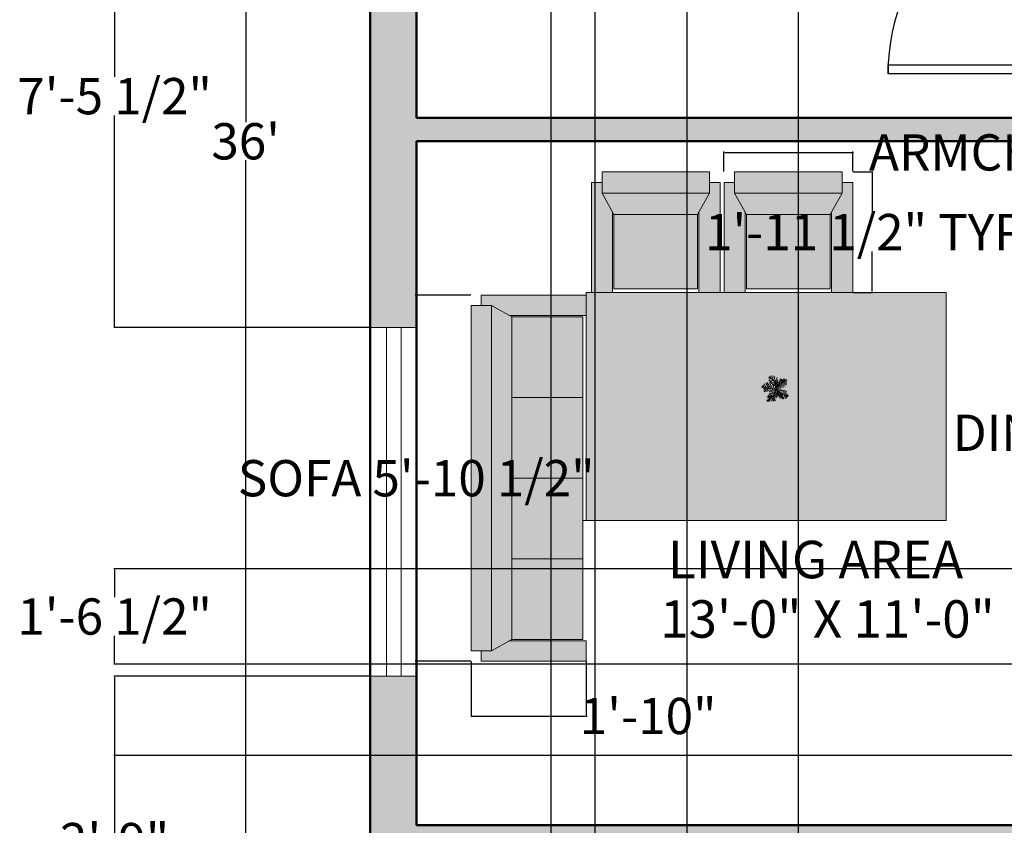
# Model space of a CAD drawing. Units: inches. Extents: x 2974 to 3443, y 2405 to 2963.
# Tile 2 of 13: x 2975 to 3165, y 2555 to 2711. Entities that reach past the tile are written whole.
import ezdxf

# ---------------------------------------------------------------- set-up
doc = ezdxf.new("R2010")
doc.units = ezdxf.units.IN
doc.header["$MEASUREMENT"] = 0
doc.layers.get('0').update_dxf_attribs({"color": 251})
for name, color, linetype, lineweight in [('A-ANNO-DIMS', 2, 'Continuous', 18), ('A-AREA-IDEN', 250, 'Continuous', 25), ('A-DOOR', 32, 'Continuous', 25), ('A-WALL-PATT', 252, 'Continuous', 13), ('furniture', 32, 'Continuous', 18), ('greenary', 106, 'Continuous', 13), ('walls', 250, 'Continuous', 50), ('windows', 159, 'Continuous', 20)]:
    doc.layers.add(name, color=color, linetype=linetype, lineweight=lineweight)
doc.layers.add('A-FURN-PATT', color=254, linetype='Continuous', lineweight=13, true_color=0xfeeab9)
doc.styles.get("Standard").update_dxf_attribs({"font": 'arial.ttf'})
doc.dimstyles.get("Standard").update_dxf_attribs({"dimtxt": 7, "dimasz": 0.18, "dimexe": 0.18, "dimexo": 0.0625, "dimgap": 0.09, "dimtad": 0, "dimtih": 1, "dimtoh": 1, "dimzin": 0, "dimdsep": 46, "dimlunit": 3, "dimtxsty": 'Standard', "dimcen": 0.09, "dimadec": 0, "dimazin": 0, "dimtfac": 1, "dimtofl": 0, "dimtmove": 0, "dimatfit": 3, "dimfxl": 1, "dimtolj": 1, "dimtzin": 0, "dimarcsym": 0})

# ---------------------------------------------------------------- blocks, each defined once
blk = doc.blocks.new('*U2')
for p, q in [((0, 0), (0, -6)), ((40, 0), (40, -6))]:
    blk.add_line(p, q)
blk.add_lwpolyline([(0, 0), (0, 40), (1.75, 40), (1.75, 0)], close=True)
blk.add_arc((0, 0), 40, 0, 90)
blk = doc.blocks.new('FABRIC SOFA 4S')
at = {"layer": 'furniture'}
for p, q in [((3, 54), (34, 54)), ((3, 51), (3, 54)), ((34, 48), (34, 54)), ((0, -51), (0, 51)), ((6, 51), (0, 51)), ((6, -51), (6, 51)), ((12, 47.63), (6, 51)), ((11.14, 48), (34, 48)), ((33, 23.81), (12, 23.81)), ((33, 0), (12, 0)), ((33, -23.81), (12, -23.81)), ((6, -51), (12, -47.63)), ((11.54, -48), (34, -48)), ((34, -48), (34, -54)), ((6, -51), (0, -51)), ((3, -54), (3, -51)), ((3, -54), (34, -54))]:
    blk.add_line(p, q, dxfattribs=at)
blk.add_lwpolyline([(12, -47.63), (12, 47.63), (33, 47.63), (33, -47.63)], close=True, dxfattribs=at)
blk = doc.blocks.new('FABRIC SOFA 1S')
at = {"layer": 'furniture'}
for p, q in [((3, 18.12), (34, 18.12)), ((3, 15.12), (3, 18.12)), ((34, 12.12), (34, 18.12)), ((0, -15.12), (0, 15.12)), ((6, 15.12), (0, 15.12)), ((6, -15.12), (6, 15.12)), ((12, 11.75), (6, 15.12)), ((11.33, 12.12), (34, 12.12)), ((6, -15.12), (12, -11.75)), ((11.33, -12.12), (34, -12.12)), ((34, -12.12), (34, -18.12)), ((6, -15.12), (0, -15.12)), ((3, -18.12), (3, -15.12)), ((3, -18.12), (34, -18.12))]:
    blk.add_line(p, q, dxfattribs=at)
blk.add_lwpolyline([(12, -11.75), (12, 11.75), (33, 11.75), (33, -11.75)], close=True, dxfattribs=at)
blk = doc.blocks.new('*U13')
for p, q in [((-5.114, 28.097), (-24.676, 40.636)), ((-7.288, 39.707), (-21.778, 46.673)), ((-8.737, 47.138), (-17.069, 52.711)), ((-10.186, 53.64), (-13.084, 55.962)), ((0, 0), (-10.5, 57)), ((-9.099, 51.782), (-6.563, 55.962)), ((-7.65, 43.423), (-2.578, 49.46)), ((-5.839, 35.992), (4.667, 48.067)), ((-5.114, 27.632), (10.463, 46.673)), ((-47.498, 19.737), (-55.83, 18.344)), ((-40.615, 13.7), (-55.105, 10.913)), ((-31.5, 4.5), (-52.5, 25.5)), ((-33.37, 6.269), (-52.207, 5.34)), ((-48.585, 21.131), (-49.309, 29.026)), ((-28.299, 3.483), (-47.86, -5.805)), ((-43.513, 28.561), (-42.427, 15.558)), ((-38.442, 26.239), (-34.819, 7.663)), ((-21.416, 3.018), (-38.079, -8.128)), ((-35.544, 28.097), (-24.314, 3.947)), ((0, 0), (-31.5, 4.5)), ((-14.533, 2.09), (-30.834, 25.31)), ((-15.982, 2.09), (-30.11, -9.521)), ((-3.665, 19.273), (-27.574, 35.527)), ((-24.314, 23.917), (-2.941, 13.7)), ((0, 0), (-22.5, -19.5)), ((-6.563, 1.161), (-21.416, -8.128)), ((-20.691, 13.7), (-1.129, 4.876)), ((-2.941, 16.486), (8.652, 37.85)), ((-1.129, 6.734), (9.014, 26.704)), ((0, 0), (27, 9)), ((0, 0), (18, -22.5)), ((3.942, 1.625), (11.187, 24.381)), ((6.478, 1.625), (26.04, -8.592)), ((10.101, 3.483), (17.708, 26.239)), ((11.187, 3.483), (30.749, -5.805)), ((16.259, 5.805), (23.142, 31.348)), ((18.07, 5.805), (35.096, -3.483)), ((22.055, 7.198), (27.489, 32.277)), ((24.229, 7.663), (46.688, 1.625)), ((27, 9), (48, 36)), ((27.127, 9.056), (31.112, 35.992)), ((29.662, 12.307), (48.137, 6.269)), ((31.836, 30.883), (32.561, 16.486)), ((33.285, 16.486), (48.862, 10.913)), ((35.096, 32.741), (37.27, 22.524)), ((36.183, 19.737), (48.137, 17.88)), ((38.719, 34.134), (41.979, 28.561)), ((40.53, 25.775), (48.862, 24.846)), ((43.791, 29.954), (51.036, 30.883)), ((44.153, 36.456), (45.239, 32.741)), ((-17.431, -15.094), (-42.789, -18.809)), ((-28.299, -29.026), (-42.789, -31.348)), ((-24.314, -21.596), (-42.427, -22.06)), ((-30.834, -34.135), (-42.427, -35.528)), ((-34.457, -39.708), (-40.978, -42.494)), ((-26.849, -26.24), (-40.253, -25.775)), ((-22.5, -19.5), (-37.5, -45)), ((-32.646, -36.921), (-31.921, -44.352)), ((-15.257, -12.772), (-30.11, -12.772)), ((-29.023, -30.884), (-27.936, -43.887)), ((-25.038, -23.918), (-22.865, -45.281)), ((-20.691, -18.345), (-17.793, -44.352)), ((-6.563, -5.805), (-19.967, -9.985)), ((-17.069, -15.094), (-12.721, -40.172)), ((-13.446, -11.378), (-8.737, -32.741)), ((-9.461, -8.592), (-6.201, -23.453)), ((-4.752, -3.483), (-3.665, -14.629)), ((2.493, -3.019), (-1.491, -20.202)), ((1.769, -2.555), (24.229, -9.521)), ((5.029, -6.27), (2.131, -25.775)), ((9.014, -11.378), (3.58, -35.992)), ((14.085, -16.951), (6.478, -40.172)), ((7.565, -9.056), (32.198, -14.629)), ((18.07, -22.524), (8.289, -45.745)), ((12.274, -15.094), (36.907, -18.809)), ((20.244, -30.419), (15.897, -44.816)), ((16.259, -19.738), (36.183, -22.989)), ((18, -22.5), (27, -52.5)), ((18.433, -22.524), (40.53, -29.026)), ((19.157, -25.311), (38.719, -33.206)), ((22.78, -37.85), (19.519, -48.532)), ((21.331, -32.741), (39.081, -40.636)), ((22.78, -38.314), (34.372, -44.816)), ((24.591, -45.745), (23.142, -50.854)), ((24.591, -43.423), (30.749, -47.603)), ((26.764, -49.925), (28.213, -50.854))]:
    blk.add_line(p, q)
blk = doc.blocks.new('*D20')
at = {"layer": 'A-ANNO-DIMS', "color": 0, "lineweight": -2, "transparency": 16777216}
for p, q in [((3018.41, 2903.19), (3018.14, 2903.19)), ((3018.32, 2903.01), (3018.32, 2690.85)), ((3018.32, 2471.37), (3018.32, 2683.52)), ((3018.41, 2471.19), (3018.14, 2471.19))]:
    blk.add_line(p, q, dxfattribs=at)
at = {"layer": 'A-ANNO-DIMS', "color": 0, "transparency": 16777216}
for points in [[(3018.29, 2903.01), (3018.35, 2903.01), (3018.32, 2903.19)], [(3018.29, 2471.37), (3018.35, 2471.37), (3018.32, 2471.19)]]:
    blk.add_solid(points, dxfattribs=at)
at = {"layer": 'Defpoints', "color": 0, "transparency": 16777216}
for p in [(3018.47, 2903.19), (3018.32, 2471.19), (3018.47, 2471.19)]:
    blk.add_point(p, dxfattribs=at)
at = {"layer": 'A-ANNO-DIMS', "color": 0, "transparency": 16777216, "insert": (3018.32, 2687.19), "char_height": 7, "attachment_point": 5}
blk.add_mtext("\\A1;36'", dxfattribs=at)
blk = doc.blocks.new('WIN-67IN')
for p, q in [((0, 0), (9, 0)), ((0, -67.29), (0, 0)), ((0, 0), (3.19, 0)), ((3.19, 0), (3.19, -67.29)), ((6.02, -67.29), (6.02, 0)), ((9, 0), (9, -67.29)), ((9, -67.29), (0, -67.29)), ((3.19, -67.29), (6.02, -67.29))]:
    blk.add_line(p, q)
blk = doc.blocks.new('*D35')
at = {"layer": 'A-ANNO-DIMS', "color": 0, "lineweight": -2, "transparency": 16777216}
for p, q in [((3110.66, 2681.38), (3110.66, 2685.22)), ((3110.84, 2685.04), (3135.33, 2685.04)), ((3135.51, 2681.38), (3135.51, 2685.22)), ((3135.51, 2685.04), (3135.69, 2685.04))]:
    blk.add_line(p, q, dxfattribs=at)
at = {"layer": 'A-ANNO-DIMS', "color": 0, "transparency": 16777216}
for points in [[(3110.84, 2685.07), (3110.84, 2685.01), (3110.66, 2685.04)], [(3135.33, 2685.07), (3135.33, 2685.01), (3135.51, 2685.04)]]:
    blk.add_solid(points, dxfattribs=at)
at = {"layer": 'Defpoints', "color": 0, "transparency": 16777216}
for p in [(3135.51, 2685.04), (3110.66, 2681.32), (3135.51, 2681.32)]:
    blk.add_point(p, dxfattribs=at)
at = {"layer": 'A-ANNO-DIMS', "color": 0, "transparency": 16777216, "insert": (3184.75, 2685.04), "char_height": 7, "attachment_point": 5}
blk.add_mtext('\\A1;ARMCHAIR 2\'-1" TYP.', dxfattribs=at)
blk = doc.blocks.new('*D36')
at = {"layer": 'A-ANNO-DIMS', "color": 0, "lineweight": -2, "transparency": 16777216}
for p, q in [((3135.57, 2681.32), (3139.42, 2681.32)), ((3139.24, 2681.14), (3139.24, 2673.37)), ((3139.24, 2658.19), (3139.24, 2665.95)), ((3135.57, 2658.01), (3139.42, 2658.01))]:
    blk.add_line(p, q, dxfattribs=at)
at = {"layer": 'A-ANNO-DIMS', "color": 0, "transparency": 16777216}
for points in [[(3139.21, 2681.14), (3139.27, 2681.14), (3139.24, 2681.32)], [(3139.21, 2658.19), (3139.27, 2658.19), (3139.24, 2658.01)]]:
    blk.add_solid(points, dxfattribs=at)
at = {"layer": 'Defpoints', "color": 0, "transparency": 16777216}
for p in [(3135.51, 2681.32), (3135.51, 2658.01), (3139.24, 2658.01)]:
    blk.add_point(p, dxfattribs=at)
at = {"layer": 'A-ANNO-DIMS', "color": 0, "transparency": 16777216, "insert": (3139.24, 2669.66), "char_height": 7, "attachment_point": 5}
blk.add_mtext('\\A1;1\'-11 1/2" TYP.', dxfattribs=at)
blk = doc.blocks.new('*D47')
at = {"layer": 'A-ANNO-DIMS', "color": 0, "lineweight": -2, "transparency": 16777216}
for p, q in [((3247.43, 2644.02), (3247.43, 2630.76)), ((3334.99, 2644.02), (3334.99, 2630.76)), ((3247.43, 2630.94), (3247.25, 2630.94)), ((3334.81, 2630.94), (3247.61, 2630.94))]:
    blk.add_line(p, q, dxfattribs=at)
at = {"layer": 'A-ANNO-DIMS', "color": 0, "transparency": 16777216}
for points in [[(3247.61, 2630.97), (3247.61, 2630.91), (3247.43, 2630.94)], [(3334.81, 2630.97), (3334.81, 2630.91), (3334.99, 2630.94)]]:
    blk.add_solid(points, dxfattribs=at)
at = {"layer": 'Defpoints', "color": 0, "transparency": 16777216}
for p in [(3247.43, 2644.08), (3334.99, 2644.08), (3247.43, 2630.94)]:
    blk.add_point(p, dxfattribs=at)
at = {"layer": 'A-ANNO-DIMS', "color": 0, "transparency": 16777216, "insert": (3200.53, 2630.94), "char_height": 7, "attachment_point": 5}
blk.add_mtext('\\A1;DINING SET 7\'-3 1/2"', dxfattribs=at)
blk = doc.blocks.new('*D49')
at = {"layer": 'A-ANNO-DIMS', "color": 0, "lineweight": -2, "transparency": 16777216}
for p, q in [((3061.77, 2657.48), (3051.06, 2657.48)), ((3051.24, 2657.3), (3051.24, 2625.89)), ((3051.24, 2587.05), (3051.24, 2618.46)), ((3061.77, 2586.87), (3051.06, 2586.87))]:
    blk.add_line(p, q, dxfattribs=at)
at = {"layer": 'A-ANNO-DIMS', "color": 0, "transparency": 16777216}
for points in [[(3051.21, 2657.3), (3051.27, 2657.3), (3051.24, 2657.48)], [(3051.21, 2587.05), (3051.27, 2587.05), (3051.24, 2586.87)]]:
    blk.add_solid(points, dxfattribs=at)
at = {"layer": 'Defpoints', "color": 0, "transparency": 16777216}
for p in [(3061.83, 2657.48), (3051.24, 2586.87), (3061.83, 2586.87)]:
    blk.add_point(p, dxfattribs=at)
at = {"layer": 'A-ANNO-DIMS', "color": 0, "transparency": 16777216, "insert": (3051.24, 2622.17), "char_height": 7, "attachment_point": 5}
blk.add_mtext('\\A1;SOFA 5\'-10 1/2"', dxfattribs=at)
blk = doc.blocks.new('*D50')
at = {"layer": 'A-ANNO-DIMS', "color": 0, "lineweight": -2, "transparency": 16777216}
for p, q in [((3061.83, 2586.81), (3061.83, 2576.1)), ((3084.06, 2586.81), (3084.06, 2576.1)), ((3062.01, 2576.28), (3083.88, 2576.28)), ((3084.06, 2576.28), (3084.24, 2576.28))]:
    blk.add_line(p, q, dxfattribs=at)
at = {"layer": 'A-ANNO-DIMS', "color": 0, "transparency": 16777216}
for points in [[(3062.01, 2576.31), (3062.01, 2576.25), (3061.83, 2576.28)], [(3083.88, 2576.31), (3083.88, 2576.25), (3084.06, 2576.28)]]:
    blk.add_solid(points, dxfattribs=at)
at = {"layer": 'Defpoints', "color": 0, "transparency": 16777216}
for p in [(3061.83, 2586.87), (3084.06, 2586.87), (3084.06, 2576.28)]:
    blk.add_point(p, dxfattribs=at)
at = {"layer": 'A-ANNO-DIMS', "color": 0, "transparency": 16777216, "insert": (3096.02, 2576.28), "char_height": 7, "attachment_point": 5}
blk.add_mtext('\\A1;1\'-10"', dxfattribs=at)
blk = doc.blocks.new('*D54')
at = {"layer": 'A-ANNO-DIMS', "color": 0, "lineweight": -2, "transparency": 16777216}
for p, q in [((3042.26, 2583.94), (2992.84, 2583.94)), ((2993.02, 2583.76), (2993.02, 2531.23)), ((2993.02, 2471.37), (2993.02, 2523.9)), ((3042.26, 2471.19), (2992.84, 2471.19))]:
    blk.add_line(p, q, dxfattribs=at)
at = {"layer": 'A-ANNO-DIMS', "color": 0, "transparency": 16777216}
for points in [[(2992.99, 2583.76), (2993.05, 2583.76), (2993.02, 2583.94)], [(2992.99, 2471.37), (2993.05, 2471.37), (2993.02, 2471.19)]]:
    blk.add_solid(points, dxfattribs=at)
at = {"layer": 'Defpoints', "color": 0, "transparency": 16777216}
for p in [(2993.02, 2583.94), (3042.33, 2583.94), (3042.33, 2471.19)]:
    blk.add_point(p, dxfattribs=at)
at = {"layer": 'A-ANNO-DIMS', "color": 0, "transparency": 16777216, "insert": (2993.02, 2527.57), "char_height": 7, "attachment_point": 5}
blk.add_mtext('\\A1;9\'-5"', dxfattribs=at)
blk = doc.blocks.new('*D55')
at = {"layer": 'A-ANNO-DIMS', "color": 0, "lineweight": -2, "transparency": 16777216}
for p, q in [((3042.26, 2740.57), (2992.84, 2740.57)), ((2993.02, 2740.39), (2993.02, 2699.61)), ((2993.02, 2651.41), (2993.02, 2692.19)), ((3042.26, 2651.23), (2992.84, 2651.23))]:
    blk.add_line(p, q, dxfattribs=at)
at = {"layer": 'A-ANNO-DIMS', "color": 0, "transparency": 16777216}
for points in [[(2992.99, 2740.39), (2993.05, 2740.39), (2993.02, 2740.57)], [(2992.99, 2651.41), (2993.05, 2651.41), (2993.02, 2651.23)]]:
    blk.add_solid(points, dxfattribs=at)
at = {"layer": 'Defpoints', "color": 0, "transparency": 16777216}
for p in [(3042.33, 2740.57), (2993.02, 2651.23), (3042.33, 2651.23)]:
    blk.add_point(p, dxfattribs=at)
at = {"layer": 'A-ANNO-DIMS', "color": 0, "transparency": 16777216, "insert": (2993.02, 2695.9), "char_height": 7, "attachment_point": 5}
blk.add_mtext('\\A1;7\'-5 1/2"', dxfattribs=at)
blk = doc.blocks.new('*D64')
at = {"layer": 'A-ANNO-DIMS', "color": 0, "lineweight": -2, "transparency": 16777216}
for p, q in [((3103.48, 2840.13), (3103.48, 2414.92)), ((3124.99, 2840.13), (3124.99, 2414.92)), ((3103.66, 2415.1), (3124.81, 2415.1)), ((3124.99, 2415.1), (3125.17, 2415.1))]:
    blk.add_line(p, q, dxfattribs=at)
at = {"layer": 'A-ANNO-DIMS', "color": 0, "transparency": 16777216}
for points in [[(3103.66, 2415.13), (3103.66, 2415.07), (3103.48, 2415.1)], [(3124.81, 2415.13), (3124.81, 2415.07), (3124.99, 2415.1)]]:
    blk.add_solid(points, dxfattribs=at)
at = {"layer": 'Defpoints', "color": 0, "transparency": 16777216}
for p in [(3103.48, 2840.19), (3124.99, 2840.19), (3124.99, 2415.1)]:
    blk.add_point(p, dxfattribs=at)
at = {"layer": 'A-ANNO-DIMS', "color": 0, "transparency": 16777216, "insert": (3142.39, 2415.1), "char_height": 7, "attachment_point": 5}
blk.add_mtext('\\A1;1\'-9 1/2"', dxfattribs=at)
blk = doc.blocks.new('*D68')
at = {"layer": 'A-ANNO-DIMS', "color": 0, "lineweight": -2, "transparency": 16777216}
for p, q in [((3077.27, 2480.25), (3077.27, 2952.68)), ((3077.45, 2952.5), (3085.63, 2952.5)), ((3085.81, 2480.25), (3085.81, 2952.68)), ((3085.81, 2952.5), (3085.99, 2952.5))]:
    blk.add_line(p, q, dxfattribs=at)
at = {"layer": 'A-ANNO-DIMS', "color": 0, "transparency": 16777216}
for points in [[(3077.45, 2952.53), (3077.45, 2952.47), (3077.27, 2952.5)], [(3085.63, 2952.53), (3085.63, 2952.47), (3085.81, 2952.5)]]:
    blk.add_solid(points, dxfattribs=at)
at = {"layer": 'Defpoints', "color": 0, "transparency": 16777216}
for p in [(3085.81, 2952.5), (3077.27, 2480.19), (3085.81, 2480.19)]:
    blk.add_point(p, dxfattribs=at)
at = {"layer": 'A-ANNO-DIMS', "color": 0, "transparency": 16777216, "insert": (3103.54, 2952.5), "char_height": 7, "attachment_point": 5}
blk.add_mtext('\\A1;0\'-8 1/2"', dxfattribs=at)
blk = doc.blocks.new('*D73')
at = {"layer": 'A-ANNO-DIMS', "color": 0, "lineweight": -2, "transparency": 16777216}
for p, q in [((3329.94, 2604.69), (2992.84, 2604.69)), ((2993.02, 2604.51), (2993.02, 2599.19)), ((2993.02, 2586.45), (2993.02, 2591.77)), ((3330, 2586.27), (2992.84, 2586.27))]:
    blk.add_line(p, q, dxfattribs=at)
at = {"layer": 'A-ANNO-DIMS', "color": 0, "transparency": 16777216}
for points in [[(2992.99, 2604.51), (2993.05, 2604.51), (2993.02, 2604.69)], [(2992.99, 2586.45), (2993.05, 2586.45), (2993.02, 2586.27)]]:
    blk.add_solid(points, dxfattribs=at)
at = {"layer": 'Defpoints', "color": 0, "transparency": 16777216}
for p in [(2993.02, 2604.69), (3330, 2604.69), (3330.06, 2586.27)]:
    blk.add_point(p, dxfattribs=at)
at = {"layer": 'A-ANNO-DIMS', "color": 0, "transparency": 16777216, "insert": (2993.02, 2595.48), "char_height": 7, "attachment_point": 5}
blk.add_mtext('\\A1;1\'-6 1/2"', dxfattribs=at)
blk = doc.blocks.new('*D76')
at = {"layer": 'A-ANNO-DIMS', "color": 0, "lineweight": -2, "transparency": 16777216}
for p, q in [((3352.84, 2568.64), (2992.84, 2568.64)), ((2993.02, 2568.46), (2993.02, 2555.8)), ((2993.02, 2535.82), (2993.02, 2548.48)), ((3352.84, 2535.64), (2992.84, 2535.64))]:
    blk.add_line(p, q, dxfattribs=at)
at = {"layer": 'A-ANNO-DIMS', "color": 0, "transparency": 16777216}
for points in [[(2992.99, 2568.46), (2993.05, 2568.46), (2993.02, 2568.64)], [(2992.99, 2535.82), (2993.05, 2535.82), (2993.02, 2535.64)]]:
    blk.add_solid(points, dxfattribs=at)
at = {"layer": 'Defpoints', "color": 0, "transparency": 16777216}
for p in [(2993.02, 2568.64), (3352.9, 2568.64), (3352.9, 2535.64)]:
    blk.add_point(p, dxfattribs=at)
at = {"layer": 'A-ANNO-DIMS', "color": 0, "transparency": 16777216, "insert": (2993.02, 2552.14), "char_height": 7, "attachment_point": 5}
blk.add_mtext('\\A1;2\'-9"', dxfattribs=at)

msp = doc.modelspace()

# ---------------------------------------------------------------- hatches: boundary and pattern name
at = {"layer": 'A-FURN-PATT'}
h = msp.add_hatch(color=256, dxfattribs=at)
h.dxf.hatch_style = 1
h.paths.add_polyline_path([(3105.53, 2673.089), (3089.42, 2673.089), (3089.42, 2658.693), (3105.53, 2658.693)])
h.paths.add_polyline_path([(3089.163, 2673.546), (3087.106, 2677.202), (3087.106, 2679.259), (3085.05, 2679.259), (3085.05, 2658.007), (3089.163, 2658.007)])
h.paths.add_polyline_path([(3109.901, 2679.259), (3107.844, 2679.259), (3107.844, 2677.202), (3105.787, 2673.546), (3105.787, 2658.007), (3109.901, 2658.007)])
h.paths.add_polyline_path([(3107.844, 2681.315), (3087.106, 2681.315), (3087.106, 2677.202), (3107.844, 2677.202)])
h = msp.add_hatch(color=256, dxfattribs=at)
h.dxf.hatch_style = 1
h.paths.add_polyline_path([(3114.771, 2673.546), (3112.715, 2677.202), (3112.715, 2679.259), (3110.658, 2679.259), (3110.658, 2658.007), (3114.771, 2658.007)])
h.paths.add_polyline_path([(3135.509, 2679.259), (3133.452, 2679.259), (3133.452, 2677.202), (3131.396, 2673.546), (3131.396, 2658.007), (3135.509, 2658.007)])
h.paths.add_polyline_path([(3133.452, 2681.315), (3112.715, 2681.315), (3112.715, 2677.202), (3133.452, 2677.202)])
h.paths.add_polyline_path([(3131.139, 2673.089), (3115.028, 2673.089), (3115.028, 2658.693), (3131.139, 2658.693)])
h = msp.add_hatch(color=256, dxfattribs=at)
h.dxf.hatch_style = 1
h.paths.add_polyline_path([(3107.844, 2677.202), (3087.106, 2677.202), (3089.42, 2673.089), (3105.53, 2673.089)])
h = msp.add_hatch(color=256, dxfattribs=at)
h.dxf.hatch_style = 1
h.paths.add_polyline_path([(3133.452, 2677.202), (3112.715, 2677.202), (3115.028, 2673.089), (3131.139, 2673.089)])
h = msp.add_hatch(color=256, dxfattribs=at)
h.dxf.hatch_style = 1
h.paths.add_polyline_path([(3083.406, 2653.31), (3069.676, 2653.31), (3069.676, 2637.742), (3083.406, 2637.742)], flags=17)
h.paths.add_polyline_path([(3083.406, 2637.742), (3069.676, 2637.742), (3069.676, 2622.173), (3083.406, 2622.173)], flags=17)
h.paths.add_polyline_path([(3083.406, 2622.173), (3069.676, 2622.173), (3069.676, 2606.605), (3083.406, 2606.605)], flags=17)
h.paths.add_polyline_path([(3083.406, 2606.605), (3069.676, 2606.605), (3069.676, 2591.036), (3083.406, 2591.036)], flags=17)
h.paths.add_polyline_path([(3084.06, 2590.791), (3069.24, 2590.791), (3065.753, 2588.83), (3063.792, 2588.83), (3063.792, 2586.869), (3084.06, 2586.869)], flags=17)
h.paths.add_polyline_path([(3065.753, 2655.517), (3061.831, 2655.517), (3061.831, 2588.83), (3065.753, 2588.83)], flags=17)
h.paths.add_polyline_path([(3069.676, 2653.31), (3083.406, 2653.31), (3083.406, 2637.742), (3069.676, 2637.742), (3069.676, 2653.31), (3065.753, 2655.517), (3065.753, 2588.83), (3069.24, 2590.791), (3084.06, 2590.791), (3084.06, 2586.869), (3063.792, 2586.869), (3063.792, 2588.83), (3061.831, 2588.83), (3061.831, 2655.517), (3063.792, 2655.517), (3063.792, 2657.478), (3084.06, 2657.478), (3084.06, 2653.556), (3069.24, 2653.556)])
h = msp.add_hatch(color=256, dxfattribs=at)
h.dxf.hatch_style = 1
h.paths.add_polyline_path([(3153.538, 2658.007), (3084.06, 2658.007), (3084.06, 2657.478), (3084.06, 2653.556), (3084.06, 2614.015), (3153.538, 2614.015)])
h = msp.add_hatch(color=256, dxfattribs=at)
h.dxf.hatch_style = 1
h.paths.add_polyline_path([(3065.753, 2655.517), (3061.831, 2655.517), (3061.831, 2588.83), (3065.753, 2588.83)])
h.paths.add_polyline_path([(3084.06, 2590.791), (3069.24, 2590.791), (3065.753, 2588.83), (3063.792, 2588.83), (3063.792, 2586.869), (3084.06, 2586.869)])
h = msp.add_hatch(color=256, dxfattribs=at)
h.dxf.hatch_style = 1
h.paths.add_polyline_path([(3069.676, 2653.31), (3065.753, 2655.517), (3065.753, 2588.83), (3069.676, 2591.036)])
h = msp.add_hatch(color=256, dxfattribs=at)
h.dxf.hatch_style = 1
h.paths.add_polyline_path([(3083.406, 2653.31), (3069.676, 2653.31), (3069.676, 2637.742), (3083.406, 2637.742)])
h = msp.add_hatch(color=256, dxfattribs=at)
h.dxf.hatch_style = 1
h.paths.add_polyline_path([(3107.334, 2631.966), (3107.334, 2643.26), (3114.459, 2643.26), (3114.459, 2645.454), (3107.334, 2645.454), (3107.334, 2647.491), (3135.026, 2647.491), (3135.026, 2637.101), (3127.556, 2637.101), (3127.556, 2634.907), (3135.026, 2634.907), (3135.026, 2631.966)])
h.paths.add_polyline_path([(3120.546, 2640.008), (3120.509, 2640.034), (3120.537, 2640.068)], flags=16)
h.paths.add_polyline_path([(3119.62, 2641.623), (3120.347, 2640.896), (3120.35, 2640.955), (3120.272, 2640.971), (3119.705, 2641.538), (3119.717, 2641.614)], flags=16)
h.paths.add_polyline_path([(3122.45, 2638.246), (3122.455, 2638.248), (3122.457, 2638.244)], flags=16)
h.paths.add_polyline_path([(3119.322, 2639.551), (3119.335, 2639.562), (3120.644, 2639.321), (3120.485, 2638.844), (3120.458, 2638.835), (3120.472, 2638.805), (3120.218, 2638.042), (3119.879, 2637.778), (3119.851, 2637.78), (3119.857, 2637.762), (3120.209, 2638.035), (3120.216, 2638.036), (3120.644, 2639.321), (3120.77, 2639.219), (3120.776, 2639.2), (3120.791, 2639.203), (3121.357, 2638.75), (3121.375, 2638.63), (3121.469, 2638.661), (3121.703, 2638.474), (3121.706, 2638.463), (3121.712, 2638.466), (3120.644, 2639.321), (3121.346, 2640.131), (3121.356, 2640.129), (3121.358, 2640.145), (3120.644, 2639.321), (3119.312, 2639.566)], flags=16)
h.paths.add_polyline_path([(3108.548, 2633.721, 1), (3108.548, 2632.919, 1)], flags=16)
h = msp.add_hatch(color=256, dxfattribs=at)
h.dxf.hatch_style = 1
h.paths.add_polyline_path([(3107.334, 2643.26), (3107.334, 2645.454), (3114.459, 2645.454), (3114.459, 2643.26)])
h.paths.add_polyline_path([(3105.368, 2643.26), (3105.368, 2645.454), (3107.334, 2645.454), (3107.334, 2643.26)])
h.paths.add_polyline_path([(3127.556, 2634.907), (3127.556, 2637.101), (3135.026, 2637.101), (3135.026, 2634.907)])
h.paths.add_polyline_path([(3135.026, 2634.907), (3135.026, 2637.101), (3136.646, 2637.101), (3136.646, 2634.907)])
at = {"layer": 'A-WALL-PATT'}
h = msp.add_hatch(color=256, dxfattribs=at)
h.dxf.hatch_style = 1
h.paths.add_polyline_path([(3222.294, 2555.188), (3211.826, 2555.188), (3211.826, 2657.938), (3207.326, 2657.938), (3207.326, 2555.188), (3051.326, 2555.188), (3051.326, 2583.943), (3042.326, 2583.943), (3042.326, 2471.188), (3165.027, 2471.188), (3165.027, 2480.188), (3051.326, 2480.188), (3051.326, 2550.688), (3222.294, 2550.688)])
h.paths.add_polyline_path([(3188.326, 2700.207), (3183.826, 2700.207), (3183.826, 2691.688), (3051.326, 2691.688), (3051.326, 2740.572), (3042.326, 2740.572), (3042.326, 2651.235), (3045.517, 2651.235), (3051.326, 2651.235), (3051.326, 2687.188), (3188.326, 2687.188)])
h.paths.add_polyline_path([(3051.326, 2894.188), (3074.298, 2894.188), (3074.298, 2903.188), (3042.326, 2903.188), (3042.326, 2807.864), (3045.517, 2807.864), (3051.326, 2807.864), (3051.326, 2835.688), (3103.457, 2835.688), (3103.457, 2839.066, -0.0124729), (3103.485, 2840.188), (3051.326, 2840.188)])
h.paths.add_polyline_path([(3201.987, 2903.188), (3100.263, 2903.188), (3100.263, 2894.188), (3131.326, 2894.188), (3131.326, 2835.688), (3135.826, 2835.688), (3135.826, 2894.188), (3183.826, 2894.188), (3183.826, 2840.188), (3159.826, 2840.188), (3159.826, 2835.688), (3183.826, 2835.688), (3183.826, 2740.207), (3188.326, 2740.207), (3188.326, 2803.688), (3215.422, 2803.688), (3215.422, 2807.066, -0.0124729), (3215.45, 2808.188), (3188.326, 2808.188), (3188.326, 2894.188), (3201.987, 2894.188)])
h.paths.add_polyline_path([(3283.564, 2903.188), (3227.952, 2903.188), (3227.952, 2894.188), (3240.326, 2894.188), (3240.326, 2755.688), (3188.326, 2755.688), (3188.326, 2751.188), (3244.826, 2751.188), (3244.826, 2757.188), (3244.826, 2797.188), (3244.826, 2894.188), (3283.564, 2894.188)])
h.paths.add_polyline_path([(3384.326, 2903.188), (3346.694, 2903.188), (3346.694, 2894.188), (3375.326, 2894.188), (3375.326, 2755.688), (3284.826, 2755.688), (3284.826, 2751.188), (3375.326, 2751.188), (3375.326, 2710.653), (3378.517, 2710.653), (3384.326, 2710.653)])
h.paths.add_polyline_path([(3384.326, 2643.361), (3375.326, 2643.361), (3375.326, 2609.188), (3330.003, 2609.188), (3330.003, 2604.688), (3375.326, 2604.688), (3375.326, 2480.188), (3356.49, 2480.188), (3356.49, 2471.188), (3384.326, 2471.188)])
h.paths.add_polyline_path([(3267.326, 2609.188), (3262.826, 2609.188), (3262.826, 2555.188), (3257.429, 2555.188), (3257.429, 2550.688), (3262.826, 2550.688), (3262.826, 2471.188), (3293.36, 2471.188), (3293.36, 2480.188), (3267.326, 2480.188)])
h.paths.add_polyline_path([(3275.186, 2471.188), (3268.471, 2471.188), (3268.471, 2455.229), (3268.471, 2452.413), (3275.186, 2452.413)])
h.paths.add_polyline_path([(3156.684, 2471.188), (3149.969, 2471.188), (3149.969, 2452.413), (3156.684, 2452.413)])

# ---------------------------------------------------------------- linework, layer by layer
at = {"layer": 'furniture'}
for p, q in [((3153.538, 2658.007), (3084.06, 2658.007)), ((3084.06, 2658.007), (3084.06, 2657.478)), ((3084.06, 2657.478), (3084.06, 2614.015)), ((3153.538, 2614.015), (3153.538, 2658.007)), ((3083.406, 2614.015), (3153.538, 2614.015))]:
    msp.add_line(p, q, dxfattribs=at)
at = {"layer": 'walls'}
for p, q in [((3042.326, 2471.188), (3042.326, 2903.188)), ((3051.326, 2691.688), (3051.326, 2835.688)), ((3051.326, 2691.688), (3183.826, 2691.688)), ((3051.326, 2687.188), (3188.326, 2687.188)), ((3051.326, 2555.188), (3051.326, 2687.188)), ((3051.326, 2555.188), (3207.326, 2555.188))]:
    msp.add_line(p, q, dxfattribs=at)

# ---------------------------------------------------------------- block references
at = {"layer": 'A-DOOR', "rotation": 90}
msp.add_blockref('*U2', (3182.326, 2700.207), dxfattribs=at)
at = {"layer": 'furniture'}
for name, p, xscale, yscale, zscale, rotation in [('FABRIC SOFA 1S', (3097.475, 2681.315), 0.685544738852578, 0.685544738852578, 0.685544738852578, 270), ('FABRIC SOFA 1S', (3123.083, 2681.315), 0.685544738852578, 0.685544738852578, 0.685544738852578, 270), ('FABRIC SOFA 4S', (3061.831, 2622.173), -0.6537939928824033, 0.6537939928824033, 0.6537939928824033, 179.9999999998931)]:
    msp.add_blockref(name, p, dxfattribs=dict(at, xscale=xscale, yscale=yscale, zscale=zscale, rotation=rotation))
at = {"layer": 'greenary', "xscale": -0.0473395969371584, "yscale": 0.0473395969371584, "zscale": 0.0473395969371584, "rotation": 90}
msp.add_blockref('*U13', (3120.644, 2639.321), dxfattribs=at)
at = {"layer": 'windows'}
msp.add_blockref('WIN-67IN', (3042.326, 2651.235), dxfattribs=at)

# ---------------------------------------------------------------- texts
at = {"layer": 'A-AREA-IDEN'}
for s, p in [('LIVING AREA', (3099.843, 2602.861)), ('13\'-0" X 11\'-0"', (3098.365, 2591.392))]:
    msp.add_text(s, height=7.22716, dxfattribs=at).set_placement(p)

# ---------------------------------------------------------------- dimensions: what is measured, and where the dimension line sits
at = {"layer": 'A-ANNO-DIMS'}
for base, p1, p2, picture, middle in [((3085.81, 2952.498), (3077.267, 2480.188), (3085.81, 2480.188), '*D68', (3103.539, 2952.498)), ((3124.986, 2415.097), (3103.485, 2840.188), (3124.986, 2840.188), '*D64', (3142.386, 2415.097)), ((3084.06, 2576.277), (3061.831, 2586.869), (3084.06, 2586.869), '*D50', (3096.023, 2576.277))]:
    dim = msp.add_linear_dim(base=base, p1=p1, p2=p2, dimstyle='Standard', override={"dimdec": 1, "dimlfac": 1, "dimrnd": 0, "dimzin": 1, "dimdsep": 46, "dimlunit": 4, "dimfrac": 2}, dxfattribs=at)
    dim.commit()
    dim.dimension.update_dxf_attribs({"geometry": picture, "text_midpoint": middle})
for base, p1, p2, override, picture, middle in [((3018.319, 2471.188), (3018.469, 2903.188), (3018.469, 2471.188), {"dimclrd": 0, "dimclre": 0, "dimclrt": 0}, '*D20', (3018.319, 2687.188)), ((2993.016, 2651.235), (3042.326, 2740.572), (3042.326, 2651.235), {"dimdec": 1, "dimlfac": 1, "dimrnd": 0, "dimzin": 1, "dimdsep": 46, "dimlunit": 4, "dimfrac": 2}, '*D55', (2993.016, 2695.903)), ((2993.016, 2604.688), (3330.059, 2586.273), (3330.003, 2604.688), {"dimdec": 1, "dimlfac": 1, "dimrnd": 0, "dimzin": 1, "dimdsep": 46, "dimlunit": 4, "dimfrac": 2}, '*D73', (2993.016, 2595.481)), ((2993.016, 2583.943), (3042.326, 2471.188), (3042.326, 2583.943), {"dimdec": 1, "dimlfac": 1, "dimrnd": 0, "dimzin": 1, "dimdsep": 46, "dimlunit": 4, "dimfrac": 2}, '*D54', (2993.016, 2527.566)), ((2993.016, 2568.64), (3352.904, 2535.64), (3352.904, 2568.64), {"dimdec": 1, "dimlfac": 1, "dimrnd": 0, "dimzin": 1, "dimdsep": 46, "dimlunit": 4, "dimfrac": 2}, '*D76', (2993.016, 2552.14))]:
    dim = msp.add_linear_dim(base=base, p1=p1, p2=p2, angle=90, dimstyle='Standard', override=override, dxfattribs=at)
    dim.commit()
    dim.dimension.update_dxf_attribs({"geometry": picture, "text_midpoint": middle})
dim = msp.add_linear_dim(base=(3135.509, 2685.043), p1=(3110.658, 2681.315), p2=(3135.509, 2681.315), text='ARMCHAIR <> TYP.', dimstyle='Standard', override={"dimdec": 1, "dimlfac": 1, "dimrnd": 0, "dimzin": 1, "dimdsep": 46, "dimlunit": 4, "dimfrac": 2}, dxfattribs=at)
dim.commit()
dim.dimension.update_dxf_attribs({"geometry": '*D35', "text_midpoint": (3184.753, 2685.043)})
for base, p1, p2, angle, text, picture, middle in [((3139.237, 2658.007), (3135.509, 2681.315), (3135.509, 2658.007), 270, '<> TYP.', '*D36', (3139.237, 2669.661)), ((3051.239, 2586.869), (3061.831, 2657.478), (3061.831, 2586.869), 270, 'SOFA <>', '*D49', (3051.239, 2622.173)), ((3247.425, 2630.944), (3334.991, 2644.079), (3247.425, 2644.079), 180, 'DINING SET <>', '*D47', (3200.531, 2630.944))]:
    dim = msp.add_linear_dim(base=base, p1=p1, p2=p2, angle=angle, text=text, dimstyle='Standard', override={"dimdec": 1, "dimlfac": 1, "dimrnd": 0, "dimzin": 1, "dimdsep": 46, "dimlunit": 4, "dimfrac": 2}, dxfattribs=at)
    dim.commit()
    dim.dimension.update_dxf_attribs({"geometry": picture, "text_midpoint": middle})

doc.saveas('drawing.dxf')
